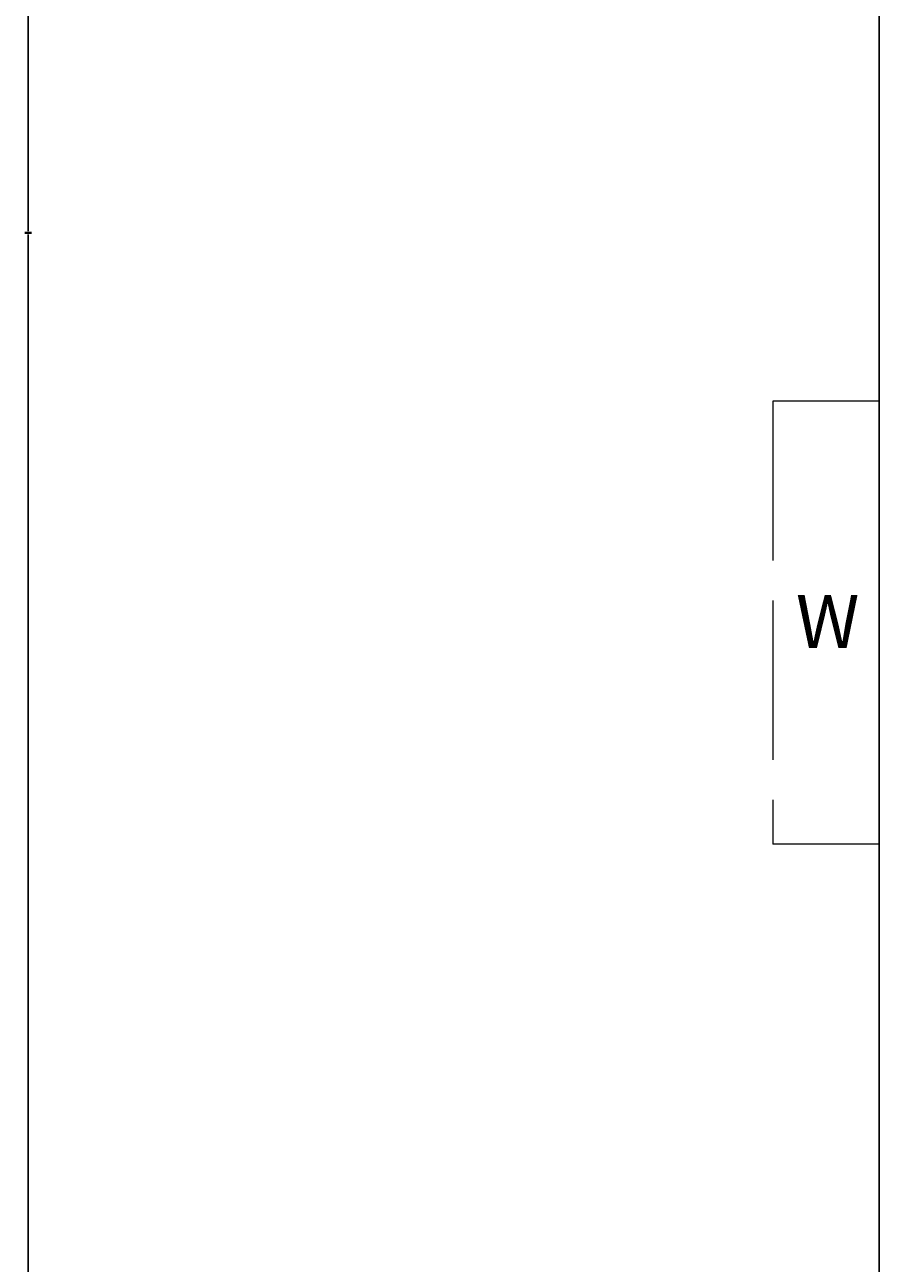
# Model space of a CAD drawing. Units: inches. Extents: x -301 to 715, y -607 to 364.
# Tile 67 of 141: x -301 to -205, y -73 to 67. Entities that reach past the tile are written whole.
import ezdxf

# ---------------------------------------------------------------- set-up
doc = ezdxf.new("R2010")
doc.units = ezdxf.units.IN
doc.header["$MEASUREMENT"] = 0
doc.linetypes.add('ACAD_ISO02W100', pattern=[15, 12, -3])
for name, color, linetype, lineweight in [('A-ANNO-DIMS', 2, 'Continuous', 18), ('A-ANNO-TEXT', 4, 'Continuous', 18), ('A-GLAZ-OVHD', 2, 'ACAD_ISO02W100', 18)]:
    doc.layers.add(name, color=color, linetype=linetype, lineweight=lineweight)
doc.styles.get("Standard").update_dxf_attribs({"font": 'arial.ttf'})
doc.dimstyles.get("Standard").update_dxf_attribs({"dimtxt": 0.18, "dimasz": 0.18, "dimexe": 0.18, "dimexo": 0.0625, "dimgap": 0.09, "dimtad": 0, "dimtih": 1, "dimtoh": 1, "dimdec": 1, "dimzin": 0, "dimdsep": 46, "dimlunit": 4, "dimtxsty": 'Standard', "dimcen": 0.09, "dimclrd": 3, "dimclre": 4, "dimclrt": 6, "dimadec": 0, "dimazin": 0, "dimtfac": 1, "dimtdec": 1, "dimtofl": 0, "dimtmove": 0, "dimatfit": 3, "dimfxl": 1, "dimtfill": 2, "dimtfillclr": 51, "dimtolj": 1, "dimtzin": 0, "dimarcsym": 0})

# ---------------------------------------------------------------- blocks, each defined once
blk = doc.blocks.new('WIN-SHADE-50')
at = {"ltscale": 1.5}
for p, q in [((0, 0), (0, 12)), ((50, 12), (0, 12)), ((50, 0), (50, 12)), ((5, 0), (0, 0)), ((45, 0), (50, 0))]:
    blk.add_line(p, q, dxfattribs=at)
blk = doc.blocks.new('*D145')
at = {"layer": 'A-ANNO-DIMS', "color": 4, "lineweight": -2, "transparency": 16777216}
for p, q in [((-204.67, 310.18), (-300.87, 310.18)), ((-204.67, -223.82), (-300.87, -223.82))]:
    blk.add_line(p, q, dxfattribs=at)
at = {"layer": 'A-ANNO-DIMS', "color": 3, "lineweight": -2, "transparency": 16777216}
for p, q in [((-300.69, 310), (-300.69, 43.36)), ((-300.69, -223.64), (-300.69, 43))]:
    blk.add_line(p, q, dxfattribs=at)
at = {"layer": 'A-ANNO-DIMS', "color": 3, "transparency": 16777216}
for points in [[(-300.72, 310), (-300.66, 310), (-300.69, 310.18)], [(-300.72, -223.64), (-300.66, -223.64), (-300.69, -223.82)]]:
    blk.add_solid(points, dxfattribs=at)
at = {"layer": 'Defpoints', "color": 0, "transparency": 16777216}
for p in [(-300.69, 310.18), (-204.6, 310.18), (-204.6, -223.82)]:
    blk.add_point(p, dxfattribs=at)
at = {"layer": 'A-ANNO-DIMS', "color": 6, "transparency": 16777216, "insert": (-300.69, 43.18), "char_height": 0.18, "attachment_point": 5, "bg_fill": 1, "box_fill_scale": 1.25, "bg_fill_color": 51, "bg_fill_transparency": 0}
blk.add_mtext('\\A1;44\'-6"', dxfattribs=at)
blk = doc.blocks.new('*D151')
at = {"layer": 'A-ANNO-DIMS', "color": 4, "lineweight": -2, "transparency": 16777216}
for p, q in [((-204.6, -223.76), (-204.6, 359.61)), ((-45.6, -214.76), (-45.6, 359.61))]:
    blk.add_line(p, q, dxfattribs=at)
at = {"layer": 'A-ANNO-DIMS', "color": 3, "lineweight": -2, "transparency": 16777216}
for p, q in [((-204.42, 359.43), (-125.49, 359.43)), ((-45.78, 359.43), (-124.71, 359.43))]:
    blk.add_line(p, q, dxfattribs=at)
at = {"layer": 'A-ANNO-DIMS', "color": 3, "transparency": 16777216}
for points in [[(-204.42, 359.46), (-204.42, 359.4), (-204.6, 359.43)], [(-45.78, 359.46), (-45.78, 359.4), (-45.6, 359.43)]]:
    blk.add_solid(points, dxfattribs=at)
at = {"layer": 'Defpoints', "color": 0, "transparency": 16777216}
for p in [(-45.6, 359.43), (-45.6, -214.82), (-204.6, -223.82)]:
    blk.add_point(p, dxfattribs=at)
at = {"layer": 'A-ANNO-DIMS', "color": 6, "transparency": 16777216, "insert": (-125.1, 359.43), "char_height": 0.18, "attachment_point": 5, "bg_fill": 1, "box_fill_scale": 1.25, "bg_fill_color": 51, "bg_fill_transparency": 0}
blk.add_mtext('\\A1;13\'-3"', dxfattribs=at)

msp = doc.modelspace()

# ---------------------------------------------------------------- block references
at = {"layer": 'A-GLAZ-OVHD', "rotation": 90.00000000000011}
msp.add_blockref('WIN-SHADE-50', (-204.6, -25.82), dxfattribs=at)

# ---------------------------------------------------------------- texts
at = {"layer": 'A-ANNO-TEXT'}
msp.add_text('W', height=6, dxfattribs=at).set_placement((-214.02, -3.69))

# ---------------------------------------------------------------- dimensions: what is measured, and where the dimension line sits
at = {"layer": 'A-ANNO-DIMS'}
dim = msp.add_linear_dim(base=(-45.6, 359.43), p1=(-204.6, -223.82), p2=(-45.6, -214.82), dimstyle='Standard', override={"dimdec": 1, "dimlfac": 1, "dimrnd": 0, "dimzin": 1, "dimdsep": 46, "dimlunit": 4, "dimfrac": 2}, dxfattribs=at)
dim.commit()
dim.dimension.update_dxf_attribs({"geometry": '*D151', "text_midpoint": (-125.1, 359.43)})
dim = msp.add_linear_dim(base=(-300.69, 310.18), p1=(-204.6, -223.82), p2=(-204.6, 310.18), angle=90, dimstyle='Standard', override={"dimdec": 1, "dimlfac": 1, "dimrnd": 0, "dimzin": 1, "dimdsep": 46, "dimlunit": 4, "dimfrac": 2}, dxfattribs=at)
dim.commit()
dim.dimension.update_dxf_attribs({"geometry": '*D145', "text_midpoint": (-300.69, 43.18)})

doc.saveas('drawing.dxf')
